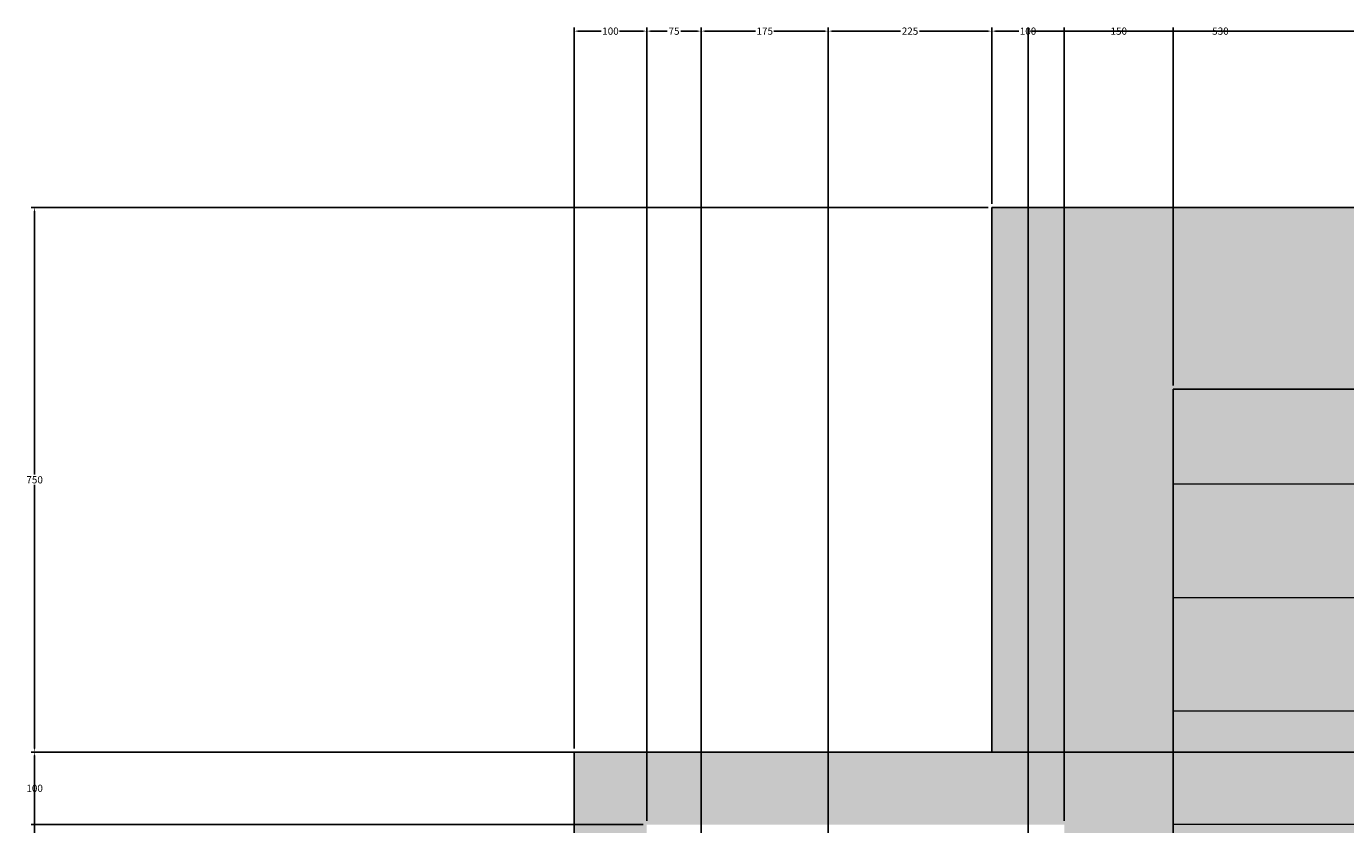
# Model space of a CAD drawing. Units: millimetres. Extents: x 2970 to 7764, y 2196 to 7505.
# Tile 8 of 13: x 2976 to 4793, y 6406 to 7505. Entities that reach past the tile are written whole.
import ezdxf

# ---------------------------------------------------------------- set-up
doc = ezdxf.new("R2010")
doc.units = ezdxf.units.MM
doc.header["$MEASUREMENT"] = 0
for name, color, linetype, lineweight in [('A-ANNO-DIMS', 2, 'Continuous', 18), ('A-ELEV', 7, 'Continuous', 25), ('A-ELEV-PATT', 8, 'Continuous', 13)]:
    doc.layers.add(name, color=color, linetype=linetype, lineweight=lineweight)
doc.styles.get("Standard").update_dxf_attribs({"font": 'arial.ttf'})
doc.dimstyles.get("Standard").update_dxf_attribs({"dimtxt": 10, "dimasz": 5, "dimexe": 5, "dimexo": 5, "dimgap": 2, "dimtad": 0, "dimtih": 1, "dimtoh": 1, "dimdec": 0, "dimzin": 0, "dimdsep": 46, "dimtxsty": 'Standard', "dimcen": 2, "dimadec": 0, "dimazin": 0, "dimtfac": 1, "dimtdec": 0, "dimtofl": 0, "dimtmove": 0, "dimatfit": 3, "dimfxl": 1, "dimtolj": 1, "dimtzin": 0, "dimarcsym": 0})

# ---------------------------------------------------------------- blocks, each defined once
blk = doc.blocks.new('*D11')
at = {"layer": 'A-ANNO-DIMS', "color": 0, "lineweight": -2, "transparency": 16777216}
for p, q in [((3730.5, 6510.8), (3730.5, 7503.8)), ((3830.5, 6410.8), (3830.5, 7503.8)), ((3735.5, 7498.8), (3767.9, 7498.8)), ((3825.5, 7498.8), (3793.1, 7498.8))]:
    blk.add_line(p, q, dxfattribs=at)
at = {"layer": 'A-ANNO-DIMS', "color": 0, "transparency": 16777216}
for points in [[(3735.5, 7499.6), (3735.5, 7498), (3730.5, 7498.8)], [(3825.5, 7499.6), (3825.5, 7498), (3830.5, 7498.8)]]:
    blk.add_solid(points, dxfattribs=at)
at = {"layer": 'Defpoints', "color": 0, "transparency": 16777216}
for p in [(3830.5, 7498.8), (3730.5, 6505.8), (3830.5, 6405.8)]:
    blk.add_point(p, dxfattribs=at)
at = {"layer": 'A-ANNO-DIMS', "color": 0, "transparency": 16777216, "insert": (3780.5, 7498.8), "char_height": 10, "attachment_point": 5}
blk.add_mtext('\\A1;100', dxfattribs=at)
blk = doc.blocks.new('*D12')
at = {"layer": 'A-ANNO-DIMS', "color": 0, "lineweight": -2, "transparency": 16777216}
for p, q in [((3830.5, 6410.8), (3830.5, 7503.8)), ((3905.5, 6260.8), (3905.5, 7503.8)), ((3835.5, 7498.8), (3858.8, 7498.8)), ((3900.5, 7498.8), (3877.2, 7498.8))]:
    blk.add_line(p, q, dxfattribs=at)
at = {"layer": 'A-ANNO-DIMS', "color": 0, "transparency": 16777216}
for points in [[(3835.5, 7499.6), (3835.5, 7498), (3830.5, 7498.8)], [(3900.5, 7499.6), (3900.5, 7498), (3905.5, 7498.8)]]:
    blk.add_solid(points, dxfattribs=at)
at = {"layer": 'Defpoints', "color": 0, "transparency": 16777216}
for p in [(3905.5, 7498.8), (3830.5, 6405.8), (3905.5, 6255.8)]:
    blk.add_point(p, dxfattribs=at)
at = {"layer": 'A-ANNO-DIMS', "color": 0, "transparency": 16777216, "insert": (3868, 7498.8), "char_height": 10, "attachment_point": 5}
blk.add_mtext('\\A1;75', dxfattribs=at)
blk = doc.blocks.new('*D13')
at = {"layer": 'A-ANNO-DIMS', "color": 0, "lineweight": -2, "transparency": 16777216}
for p, q in [((3905.5, 6260.8), (3905.5, 7503.8)), ((4080.5, 5608.3), (4080.5, 7503.8)), ((3910.5, 7498.8), (3980.4, 7498.8)), ((4075.5, 7498.8), (4005.6, 7498.8))]:
    blk.add_line(p, q, dxfattribs=at)
at = {"layer": 'A-ANNO-DIMS', "color": 0, "transparency": 16777216}
for points in [[(3910.5, 7499.6), (3910.5, 7498), (3905.5, 7498.8)], [(4075.5, 7499.6), (4075.5, 7498), (4080.5, 7498.8)]]:
    blk.add_solid(points, dxfattribs=at)
at = {"layer": 'Defpoints', "color": 0, "transparency": 16777216}
for p in [(4080.5, 7498.8), (3905.5, 6255.8), (4080.5, 5603.3)]:
    blk.add_point(p, dxfattribs=at)
at = {"layer": 'A-ANNO-DIMS', "color": 0, "transparency": 16777216, "insert": (3993, 7498.8), "char_height": 10, "attachment_point": 5}
blk.add_mtext('\\A1;175', dxfattribs=at)
blk = doc.blocks.new('*D14')
at = {"layer": 'A-ANNO-DIMS', "color": 0, "lineweight": -2, "transparency": 16777216}
for p, q in [((4080.5, 5608.3), (4080.5, 7503.8)), ((4305.5, 7260.8), (4305.5, 7503.8)), ((4085.5, 7498.8), (4179.8, 7498.8)), ((4300.5, 7498.8), (4206.2, 7498.8))]:
    blk.add_line(p, q, dxfattribs=at)
at = {"layer": 'A-ANNO-DIMS', "color": 0, "transparency": 16777216}
for points in [[(4085.5, 7499.6), (4085.5, 7498), (4080.5, 7498.8)], [(4300.5, 7499.6), (4300.5, 7498), (4305.5, 7498.8)]]:
    blk.add_solid(points, dxfattribs=at)
at = {"layer": 'Defpoints', "color": 0, "transparency": 16777216}
for p in [(4305.5, 7498.8), (4305.5, 7255.8), (4080.5, 5603.3)]:
    blk.add_point(p, dxfattribs=at)
at = {"layer": 'A-ANNO-DIMS', "color": 0, "transparency": 16777216, "insert": (4193, 7498.8), "char_height": 10, "attachment_point": 5}
blk.add_mtext('\\A1;225', dxfattribs=at)
blk = doc.blocks.new('*D15')
at = {"layer": 'A-ANNO-DIMS', "color": 0, "lineweight": -2, "transparency": 16777216}
for p, q in [((4305.5, 7260.8), (4305.5, 7503.8)), ((4405.5, 6410.8), (4405.5, 7503.8)), ((4310.5, 7498.8), (4342.9, 7498.8)), ((4400.5, 7498.8), (4368.1, 7498.8))]:
    blk.add_line(p, q, dxfattribs=at)
at = {"layer": 'A-ANNO-DIMS', "color": 0, "transparency": 16777216}
for points in [[(4310.5, 7499.6), (4310.5, 7498), (4305.5, 7498.8)], [(4400.5, 7499.6), (4400.5, 7498), (4405.5, 7498.8)]]:
    blk.add_solid(points, dxfattribs=at)
at = {"layer": 'Defpoints', "color": 0, "transparency": 16777216}
for p in [(4405.5, 7498.8), (4305.5, 7255.8), (4405.5, 6405.8)]:
    blk.add_point(p, dxfattribs=at)
at = {"layer": 'A-ANNO-DIMS', "color": 0, "transparency": 16777216, "insert": (4355.5, 7498.8), "char_height": 10, "attachment_point": 5}
blk.add_mtext('\\A1;100', dxfattribs=at)
blk = doc.blocks.new('*D16')
at = {"layer": 'A-ANNO-DIMS', "color": 0, "lineweight": -2, "transparency": 16777216}
for p, q in [((4405.5, 6410.8), (4405.5, 7503.8)), ((4555.5, 7010.8), (4555.5, 7503.8)), ((4410.5, 7498.8), (4467.9, 7498.8)), ((4550.5, 7498.8), (4493.1, 7498.8))]:
    blk.add_line(p, q, dxfattribs=at)
at = {"layer": 'A-ANNO-DIMS', "color": 0, "transparency": 16777216}
for points in [[(4410.5, 7499.6), (4410.5, 7498), (4405.5, 7498.8)], [(4550.5, 7499.6), (4550.5, 7498), (4555.5, 7498.8)]]:
    blk.add_solid(points, dxfattribs=at)
at = {"layer": 'Defpoints', "color": 0, "transparency": 16777216}
for p in [(4555.5, 7498.8), (4555.5, 7005.8), (4405.5, 6405.8)]:
    blk.add_point(p, dxfattribs=at)
at = {"layer": 'A-ANNO-DIMS', "color": 0, "transparency": 16777216, "insert": (4480.5, 7498.8), "char_height": 10, "attachment_point": 5}
blk.add_mtext('\\A1;150', dxfattribs=at)
blk = doc.blocks.new('*D17')
at = {"layer": 'A-ANNO-DIMS', "color": 0, "lineweight": -2, "transparency": 16777216}
for p, q in [((4555.5, 7010.8), (4555.5, 7503.8)), ((6155.5, 7010.8), (6155.5, 7503.8)), ((4560.5, 7498.8), (5339.1, 7498.8)), ((6150.5, 7498.8), (5371.9, 7498.8))]:
    blk.add_line(p, q, dxfattribs=at)
at = {"layer": 'A-ANNO-DIMS', "color": 0, "transparency": 16777216}
for points in [[(4560.5, 7499.6), (4560.5, 7498), (4555.5, 7498.8)], [(6150.5, 7499.6), (6150.5, 7498), (6155.5, 7498.8)]]:
    blk.add_solid(points, dxfattribs=at)
at = {"layer": 'Defpoints', "color": 0, "transparency": 16777216}
for p in [(6155.5, 7498.8), (4555.5, 7005.8), (6155.5, 7005.8)]:
    blk.add_point(p, dxfattribs=at)
at = {"layer": 'A-ANNO-DIMS', "color": 0, "transparency": 16777216, "insert": (5355.5, 7498.8), "char_height": 10, "attachment_point": 5}
blk.add_mtext('\\A1;1600', dxfattribs=at)
blk = doc.blocks.new('*D26')
at = {"layer": 'A-ANNO-DIMS', "color": 0, "lineweight": -2, "transparency": 16777216}
for p, q in [((3825.5, 6405.8), (2982.5, 6405.8)), ((2987.5, 6400.8), (2987.5, 6337.9)), ((2987.5, 6260.8), (2987.5, 6323.7)), ((3900.5, 6255.8), (2982.5, 6255.8))]:
    blk.add_line(p, q, dxfattribs=at)
at = {"layer": 'A-ANNO-DIMS', "color": 0, "transparency": 16777216}
for points in [[(2986.7, 6400.8), (2988.3, 6400.8), (2987.5, 6405.8)], [(2986.7, 6260.8), (2988.3, 6260.8), (2987.5, 6255.8)]]:
    blk.add_solid(points, dxfattribs=at)
at = {"layer": 'Defpoints', "color": 0, "transparency": 16777216}
for p in [(2987.5, 6405.8), (3830.5, 6405.8), (3905.5, 6255.8)]:
    blk.add_point(p, dxfattribs=at)
at = {"layer": 'A-ANNO-DIMS', "color": 0, "transparency": 16777216, "insert": (2987.5, 6330.8), "char_height": 10, "attachment_point": 5}
blk.add_mtext('\\A1;150', dxfattribs=at)
blk = doc.blocks.new('*D27')
at = {"layer": 'A-ANNO-DIMS', "color": 0, "lineweight": -2, "transparency": 16777216}
for p, q in [((3725.5, 6505.8), (2982.5, 6505.8)), ((2987.5, 6500.8), (2987.5, 6462.9)), ((2987.5, 6410.8), (2987.5, 6448.7)), ((3825.5, 6405.8), (2982.5, 6405.8))]:
    blk.add_line(p, q, dxfattribs=at)
at = {"layer": 'A-ANNO-DIMS', "color": 0, "transparency": 16777216}
for points in [[(2986.7, 6500.8), (2988.3, 6500.8), (2987.5, 6505.8)], [(2986.7, 6410.8), (2988.3, 6410.8), (2987.5, 6405.8)]]:
    blk.add_solid(points, dxfattribs=at)
at = {"layer": 'Defpoints', "color": 0, "transparency": 16777216}
for p in [(2987.5, 6505.8), (3730.5, 6505.8), (3830.5, 6405.8)]:
    blk.add_point(p, dxfattribs=at)
at = {"layer": 'A-ANNO-DIMS', "color": 0, "transparency": 16777216, "insert": (2987.5, 6455.8), "char_height": 10, "attachment_point": 5}
blk.add_mtext('\\A1;100', dxfattribs=at)
blk = doc.blocks.new('*D28')
at = {"layer": 'A-ANNO-DIMS', "color": 0, "lineweight": -2, "transparency": 16777216}
for p, q in [((4300.5, 7255.8), (2982.5, 7255.8)), ((2987.5, 7250.8), (2987.5, 6887.9)), ((2987.5, 6510.8), (2987.5, 6873.7)), ((3725.5, 6505.8), (2982.5, 6505.8))]:
    blk.add_line(p, q, dxfattribs=at)
at = {"layer": 'A-ANNO-DIMS', "color": 0, "transparency": 16777216}
for points in [[(2986.7, 7250.8), (2988.3, 7250.8), (2987.5, 7255.8)], [(2986.7, 6510.8), (2988.3, 6510.8), (2987.5, 6505.8)]]:
    blk.add_solid(points, dxfattribs=at)
at = {"layer": 'Defpoints', "color": 0, "transparency": 16777216}
for p in [(2987.5, 7255.8), (4305.5, 7255.8), (3730.5, 6505.8)]:
    blk.add_point(p, dxfattribs=at)
at = {"layer": 'A-ANNO-DIMS', "color": 0, "transparency": 16777216, "insert": (2987.5, 6880.8), "char_height": 10, "attachment_point": 5}
blk.add_mtext('\\A1;750', dxfattribs=at)
blk = doc.blocks.new('*D34')
at = {"layer": 'A-ANNO-DIMS', "color": 0, "lineweight": -2, "transparency": 16777216}
for p, q in [((4355.5, 4210.8), (4355.5, 7503.8)), ((4885.5, 4210.8), (4885.5, 7503.8)), ((4360.5, 7498.8), (4607.5, 7498.8)), ((4880.5, 7498.8), (4633.5, 7498.8))]:
    blk.add_line(p, q, dxfattribs=at)
at = {"layer": 'A-ANNO-DIMS', "color": 0, "transparency": 16777216}
for points in [[(4360.5, 7499.6), (4360.5, 7498), (4355.5, 7498.8)], [(4880.5, 7499.6), (4880.5, 7498), (4885.5, 7498.8)]]:
    blk.add_solid(points, dxfattribs=at)
at = {"layer": 'Defpoints', "color": 0, "transparency": 16777216}
for p in [(4885.5, 7498.8), (4355.5, 4205.8), (4885.5, 4205.8)]:
    blk.add_point(p, dxfattribs=at)
at = {"layer": 'A-ANNO-DIMS', "color": 0, "transparency": 16777216, "insert": (4620.5, 7498.8), "char_height": 10, "attachment_point": 5}
blk.add_mtext('\\A1;530', dxfattribs=at)
blk = doc.blocks.new('*D82')
at = {"layer": 'A-ANNO-DIMS', "color": 0, "lineweight": -2, "transparency": 16777216}
for p, q in [((6000.5, 6505.8), (2982.5, 6505.8)), ((2987.5, 6500.8), (2987.5, 6375.4)), ((2987.5, 6235.8), (2987.5, 6361.2)), ((6000.5, 6230.8), (2982.5, 6230.8))]:
    blk.add_line(p, q, dxfattribs=at)
at = {"layer": 'A-ANNO-DIMS', "color": 0, "transparency": 16777216}
for points in [[(2986.7, 6500.8), (2988.3, 6500.8), (2987.5, 6505.8)], [(2986.7, 6235.8), (2988.3, 6235.8), (2987.5, 6230.8)]]:
    blk.add_solid(points, dxfattribs=at)
at = {"layer": 'Defpoints', "color": 0, "transparency": 16777216}
for p in [(2987.5, 6505.8), (6005.5, 6505.8), (6005.5, 6230.8)]:
    blk.add_point(p, dxfattribs=at)
at = {"layer": 'A-ANNO-DIMS', "color": 0, "transparency": 16777216, "insert": (2987.5, 6368.3), "char_height": 10, "attachment_point": 5}
blk.add_mtext('\\A1;275', dxfattribs=at)

msp = doc.modelspace()

# ---------------------------------------------------------------- hatches: boundary and pattern name
at = {"layer": 'A-ELEV-PATT'}
h = msp.add_hatch(color=256, dxfattribs=at)
h.dxf.hatch_style = 1
h.paths.add_polyline_path([(6405.5, 7255.789), (4305.5, 7255.789), (4305.5, 6505.789), (3730.5, 6505.789), (3730.5, 4205.789), (3730.5, 2945.789), (3730.5, 2895.789), (3830.5, 2895.789), (3830.5, 4205.789), (3830.5, 6405.789), (4405.5, 6405.789), (4405.5, 4205.789), (6905.5, 4205.789), (6905.5, 2945.789), (6905.5, 2845.789), (7155.5, 2845.789), (7155.5, 2945.789), (7155.5, 4205.789), (7155.5, 4455.789), (4555.5, 4455.789), (4555.5, 6505.789), (4555.5, 7005.789), (6155.5, 7005.789), (6155.5, 6755.789), (6405.5, 6755.789)])
h.paths.add_polyline_path([(7405.5, 6755.789), (6155.5, 6755.789), (5755.5, 6755.789), (5755.5, 5005.789), (7405.5, 5005.789)])
h.paths.add_polyline_path([(7155.5, 6505.789), (7155.5, 5255.789), (6005.5, 5255.789), (6005.5, 6505.789)], flags=16)
h.paths.add_polyline_path([(6105.5, 5520.789), (6105.5, 6055.789), (6455.5, 6055.789), (6455.5, 5520.789), (6655.5, 5520.789), (6655.5, 5605.789), (6655.5, 5955.789), (6955.5, 5955.789), (6955.5, 5605.789), (6955.5, 5520.789)], flags=0)
h.paths.add_polyline_path([(6425.5, 5755.789), (6425.5, 5655.789), (6425.5, 5555.789), (6405.5, 5555.789), (6405.5, 5755.789)], flags=0)
h.paths.add_polyline_path([(6955.5, 5505.789), (6955.5, 5405.789), (6655.5, 5405.789), (6655.5, 5505.789)], flags=0)
h = msp.add_hatch(color=256, dxfattribs=at)
h.set_gradient(color1=(147, 149, 152), color2=(199, 200, 202), name='CURVED')
h.paths.add_polyline_path([(6955.5, 4455.789), (6955.5, 5005.789), (5755.5, 5005.789), (5755.5, 6755.789), (6155.5, 6755.789), (6155.5, 7005.789), (4555.5, 7005.789), (4555.5, 6505.789), (4555.5, 4455.789)])
h.paths.add_polyline_path([(5015.81, 5462.49), (5015.81, 6062.49), (5455.81, 6062.49), (5455.81, 5462.49)], flags=16)
h.paths.add_polyline_path([(5035.81, 5482.49), (5035.81, 6042.49), (5155.81, 6042.49), (5155.81, 5482.49)], flags=0)
h.paths.add_polyline_path([(5175.81, 5482.49), (5175.81, 6042.49), (5295.81, 6042.49), (5295.81, 5482.49)], flags=0)
h.paths.add_polyline_path([(5315.81, 5482.49), (5315.81, 6042.49), (5435.81, 6042.49), (5435.81, 5482.49)], flags=0)
h.paths.add_polyline_path([(4865.81, 6162.49), (4865.81, 6212.49), (4840.81, 6212.49), (4840.81, 6237.49), (5630.81, 6237.49), (5630.81, 6212.49), (5605.81, 6212.49), (5605.81, 6162.49), (5015.81, 6162.49)], flags=16)
h = msp.add_hatch(dxfattribs=at)
h.set_pattern_fill('ANSI31', color=256, scale=1250, angle=135, style=0)
h.paths.add_polyline_path([(5755.5, 6755.789), (6155.5, 6755.789), (6155.5, 7005.789), (4555.5, 7005.789), (4555.5, 6505.789), (4555.5, 4455.789), (6955.5, 4455.789), (6955.5, 5005.789), (5755.5, 5005.789)])
h.paths.add_polyline_path([(5015.81, 5462.49), (5015.81, 6062.49), (5455.81, 6062.49), (5455.81, 5462.49)], flags=16)
h.paths.add_polyline_path([(5035.81, 5482.49), (5035.81, 6042.49), (5155.81, 6042.49), (5155.81, 5482.49)], flags=0)
h.paths.add_polyline_path([(5175.81, 5482.49), (5175.81, 6042.49), (5295.81, 6042.49), (5295.81, 5482.49)], flags=0)
h.paths.add_polyline_path([(5315.81, 5482.49), (5315.81, 6042.49), (5435.81, 6042.49), (5435.81, 5482.49)], flags=0)
h.paths.add_polyline_path([(4865.81, 6162.49), (4865.81, 6212.49), (4840.81, 6212.49), (4840.81, 6237.49), (5630.81, 6237.49), (5630.81, 6212.49), (5605.81, 6212.49), (5605.81, 6162.49), (5015.81, 6162.49)], flags=16)

# ---------------------------------------------------------------- linework, layer by layer
at = {"layer": 'A-ELEV'}
for p, q in [((4305.5, 7255.789), (6405.5, 7255.789)), ((4305.5, 6505.789), (4305.5, 7255.789)), ((4555.5, 6505.789), (4555.5, 7005.789)), ((4555.5, 7005.789), (6155.5, 7005.789)), ((3730.5, 4205.789), (3730.5, 6505.789)), ((3730.5, 6505.789), (4305.5, 6505.789)), ((4555.5, 6505.789), (4555.5, 4455.789))]:
    msp.add_line(p, q, dxfattribs=at)

# ---------------------------------------------------------------- dimensions: what is measured, and where the dimension line sits
at = {"layer": 'A-ANNO-DIMS'}
for base, p1, p2, picture, middle in [((3830.5, 7498.789), (3730.5, 6505.789), (3830.5, 6405.789), '*D11', (3780.5, 7498.789)), ((3905.5, 7498.789), (3830.5, 6405.789), (3905.5, 6255.789), '*D12', (3868, 7498.789)), ((4080.5, 7498.789), (3905.5, 6255.789), (4080.5, 5603.289), '*D13', (3993, 7498.789)), ((4305.5, 7498.789), (4080.5, 5603.289), (4305.5, 7255.789), '*D14', (4193, 7498.789)), ((4405.5, 7498.789), (4305.5, 7255.789), (4405.5, 6405.789), '*D15', (4355.5, 7498.789)), ((4885.5, 7498.789), (4355.5, 4205.789), (4885.5, 4205.789), '*D34', (4620.5, 7498.789)), ((4555.5, 7498.789), (4405.5, 6405.789), (4555.5, 7005.789), '*D16', (4480.5, 7498.789)), ((6155.5, 7498.789), (4555.5, 7005.789), (6155.5, 7005.789), '*D17', (5355.5, 7498.789))]:
    dim = msp.add_linear_dim(base=base, p1=p1, p2=p2, dimstyle='Standard', override={"dimdec": 0, "dimlfac": 1, "dimrnd": 0, "dimzin": 0, "dimdsep": 46, "dimlunit": 2}, dxfattribs=at)
    dim.commit()
    dim.dimension.update_dxf_attribs({"geometry": picture, "text_midpoint": middle})
for base, p1, p2, picture, middle in [((2987.5, 7255.789), (3730.5, 6505.789), (4305.5, 7255.789), '*D28', (2987.5, 6880.789)), ((2987.5, 6505.789), (3830.5, 6405.789), (3730.5, 6505.789), '*D27', (2987.5, 6455.789)), ((2987.5, 6505.789), (6005.5, 6230.789), (6005.5, 6505.789), '*D82', (2987.5, 6368.289)), ((2987.5, 6405.789), (3905.5, 6255.789), (3830.5, 6405.789), '*D26', (2987.5, 6330.789))]:
    dim = msp.add_linear_dim(base=base, p1=p1, p2=p2, angle=90, dimstyle='Standard', override={"dimdec": 0, "dimlfac": 1, "dimrnd": 0, "dimzin": 0, "dimdsep": 46, "dimlunit": 2}, dxfattribs=at)
    dim.commit()
    dim.dimension.update_dxf_attribs({"geometry": picture, "text_midpoint": middle})

doc.saveas('drawing.dxf')
